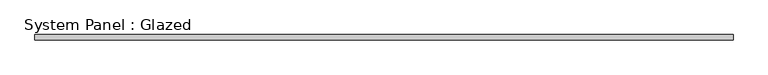
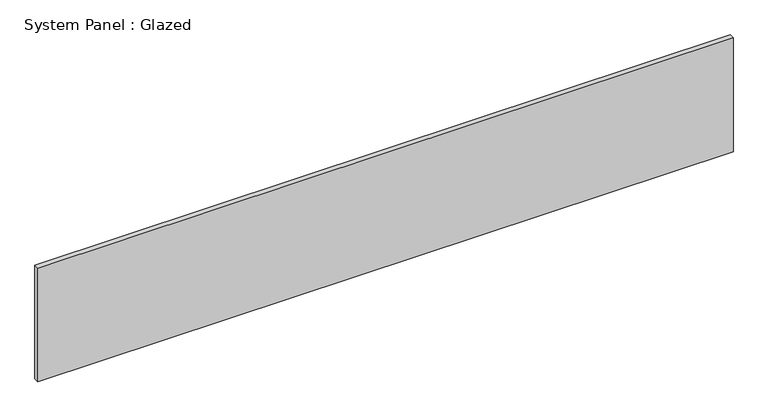
"""IFC4 building model written with IfcOpenShell, lengths in millimetres: plate geometry, System Panel : Glazed."""

from ifc_helpers import new_model, si_unit, origin, origin_with_axes, place, context, project, spatial, polyline, outline, extrude, source, transform, mapped, element, save


def system_panel_glazed_f75d5544(model_context):
    return source(origin(), model_context, "Body", "SweptSolid", [
        extrude(outline(polyline([(1691.9937474, 19.05), (-1691.9937474, 19.05), (-1691.9937474, 44.45), (1691.9937474, 44.45), (1691.9937474, 19.05)])), origin_with_axes(), (0.0, 0.0, 1.0), 585.0687666),
    ])


if __name__ == "__main__":
    model = new_model("IFC4")
    model_context = context("Model", 3, world=origin())
    ifc_project = project(units=[si_unit("LENGTHUNIT", "METRE", prefix="MILLI")], contexts=[model_context])
    site = spatial("IfcSite", under=ifc_project)
    building = spatial("IfcBuilding", under=site)
    placement = place(None, origin())
    system_panel_glazed_shape = system_panel_glazed_f75d5544(model_context)
    element("IfcPlate", 1, ObjectType="System Panel : Glazed", at=placement, inside=building, context=model_context, shape_type="MappedRepresentation", body=[
        mapped(system_panel_glazed_shape, transform((0.0, 0.0, 0.0), x_axis=(1.0, 0.0, 0.0), y_axis=(0.0, 1.0, 0.0), z_axis=(0.0, 0.0, 1.0))),
    ])
    save(model, "model.ifc")

# Revit data of these elements
# Type "System Panel : Glazed"
#   Construction Type Id = "GSP4R"
#   Analytic Construction = "1/8 in Pilkington single glazing"
#   Visual Light Transmittance = 0.9
#   Solar Heat Gain Coefficient = 0.86
#   Heat Transfer Coefficient (U) = 1.18115 BTU/(h·ft²·°F)
#   Define Thermal Properties by = 1
# Element 1 (IfcPlate, "System Panel : Glazed")
#   Materials on its faces: "Glass"
# Materials
#   "Glass": class "Glass", colour RGB 0 128 192, transparency 0.75, Description = "Soda Lime Glass", Cost = 0
